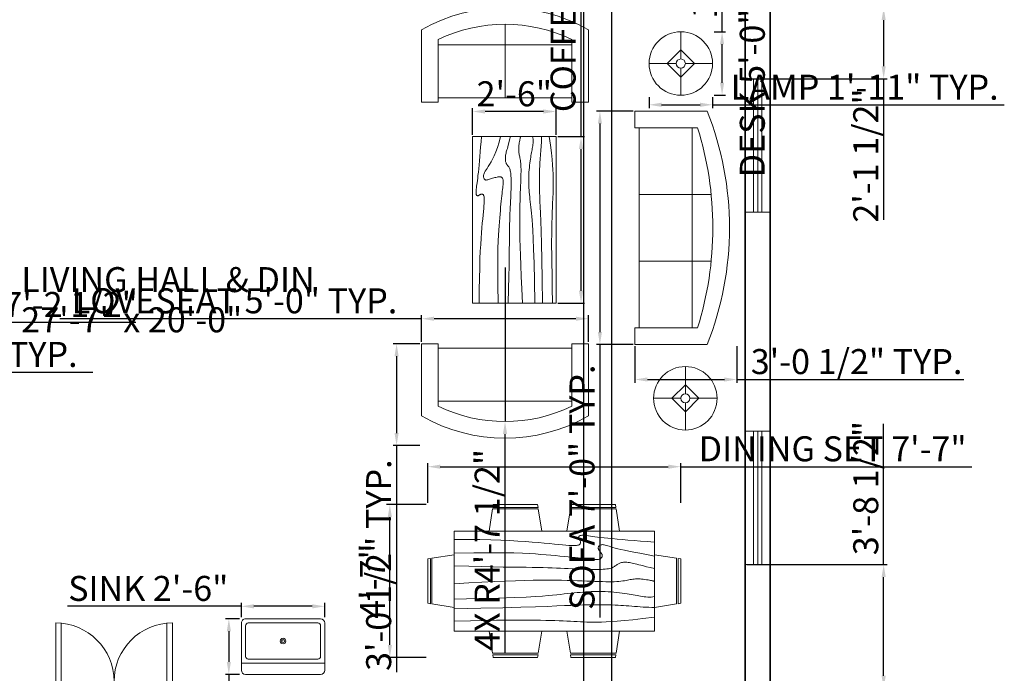
# Model space of a CAD drawing. Units: inches. Extents: x 1885 to 4781, y 1153 to 4395.
# Tile 5 of 7: x 2631 to 2985, y 1789 to 2024. Entities that reach past the tile are written whole.
import ezdxf

# ---------------------------------------------------------------- set-up
doc = ezdxf.new("R2010")
doc.units = ezdxf.units.IN
for name, color, linetype, lineweight in [('A-ANNO-DIMS', 5, 'Continuous', 18), ('A-FURN', 8, 'Continuous', 18), ('A-WALL', 7, 'Continuous', 35)]:
    doc.layers.add(name, color=color, linetype=linetype, lineweight=lineweight)
for name, color, linetype, lineweight, true_color in [('A-AREA-IDEN', 244, 'Continuous', 18, 0x991b1e), ('A-DOOR', 11, 'Continuous', 18, 0xf27172), ('A-FLOR-FIXT', 11, 'Continuous', 18, 0xf27172), ('A-GLAZ', 152, 'Continuous', 18, 0x2776bb)]:
    doc.layers.add(name, color=color, linetype=linetype, lineweight=lineweight, true_color=true_color)
doc.styles.get("Standard").update_dxf_attribs({"font": 'arial.ttf'})
doc.dimstyles.new('ISO-25', dxfattribs={"dimtxt": 9, "dimasz": 4.5, "dimexe": 1.25, "dimexo": 0.625, "dimtad": 1, "dimdec": 0, "dimlunit": 3, "dimtxsty": 'Standard', "dimcen": 2.5, "dimadec": 0, "dimazin": 0, "dimtfac": 1, "dimtdec": 0, "dimtmove": 0, "dimatfit": 3, "dimfxl": 1, "dimarcsym": 0})

# ---------------------------------------------------------------- blocks, each defined once
blk = doc.blocks.new('Table - Rectangular Woodgrain 60 x 30 in.')
for p, q in [((0, 0), (0, -30)), ((60, 0), (0, 0)), ((60, -30), (60, 0)), ((0, -30), (60, -30))]:
    blk.add_line(p, q)
for points in [[(0, -2.4), (4.8155, -2.418), (9.0302, -2.4688), (12.709, -2.5477), (15.9167, -2.65), (18.7181, -2.7711), (21.1781, -2.9063), (23.3616, -3.0508), (25.3333, -3.2), (27.1477, -3.3495), (28.8172, -3.4958), (30.3437, -3.636), (31.7291, -3.7667), (32.9756, -3.8849), (34.0849, -3.9875), (35.059, -4.0714), (35.9, -4.1334), (36.6114, -4.1711), (37.2041, -4.1854), (37.6906, -4.1779), (38.0833, -4.15), (38.3948, -4.1034), (38.6375, -4.0396), (38.8239, -3.9602), (38.9666, -3.8667), (39.0764, -3.7608), (39.1573, -3.6448), (39.2116, -3.521), (39.2416, -3.3917), (39.2498, -3.2593), (39.2385, -3.1261), (39.21, -2.9944), (39.1666, -2.8667), (39.111, -2.7447), (39.0468, -2.6281), (38.978, -2.5163), (38.9083, -2.4083), (38.8418, -2.3035), (38.7823, -2.201), (38.7337, -2.1001), (38.7, -2), (38.6844, -1.9003), (38.6875, -1.8021), (38.7094, -1.707), (38.75, -1.6167), (38.8094, -1.5326), (38.8875, -1.4563), (38.9844, -1.3893), (39.1, -1.3333), (39.2351, -1.2896), (39.3937, -1.2583), (39.5804, -1.2396), (39.8, -1.2333), (40.057, -1.2396), (40.3562, -1.2583), (40.7023, -1.2896), (41.1, -1.3333), (41.5547, -1.3895), (42.0755, -1.4573), (42.6721, -1.5361), (43.3542, -1.625), (44.1316, -1.7233), (45.014, -1.8302), (46.0114, -1.9449), (47.1333, -2.0667), (48.3862, -2.1947), (49.7625, -2.3281), (51.2513, -2.4663), (52.8416, -2.6083), (54.5226, -2.7535), (56.2833, -2.9011), (58.1127, -3.0501), (60, -3.2)], [(0, -9.2), (6.5759, -9.0858), (11.9385, -9.0365), (16.2527, -9.0418), (19.6833, -9.0917), (22.3952, -9.1759), (24.5531, -9.2844), (26.322, -9.4069), (27.8666, -9.5333), (29.3241, -9.6553), (30.7203, -9.7719), (32.0532, -9.8837), (33.3208, -9.9917), (34.5213, -10.0965), (35.6526, -10.199), (36.7128, -10.2999), (37.7, -10.4), (38.6129, -10.4996), (39.4531, -10.5969), (40.223, -10.6895), (40.925, -10.775), (41.5613, -10.8512), (42.1344, -10.9156), (42.6465, -10.966), (43.1, -11), (43.4976, -11.0158), (43.8437, -11.0136), (44.143, -10.9942), (44.4, -10.9583), (44.6195, -10.9069), (44.8062, -10.8406), (44.9648, -10.7603), (45.1, -10.6667), (45.2155, -10.5598), (45.3114, -10.4365), (45.3871, -10.2929), (45.4416, -10.125), (45.4743, -9.929), (45.4844, -9.7011), (45.4709, -9.4371), (45.4333, -9.1333), (45.3716, -8.7883), (45.2896, -8.4104), (45.1919, -8.0107), (45.0833, -7.6), (44.9685, -7.1893), (44.8521, -6.7896), (44.7388, -6.4117), (44.6333, -6.0667), (44.54, -5.7628), (44.4614, -5.4979), (44.4001, -5.2675), (44.3583, -5.0667), (44.3384, -4.8909), (44.3427, -4.7354), (44.3736, -4.5956), (44.4333, -4.4667), (44.5236, -4.3453), (44.6427, -4.2333), (44.7884, -4.1339), (44.9583, -4.05), (45.1501, -3.9849), (45.3614, -3.9417), (45.59, -3.9234), (45.8333, -3.9333), (46.0915, -3.9749), (46.3734, -4.0531), (46.6906, -4.1736), (47.0542, -4.3417), (47.4756, -4.5629), (47.9661, -4.8427), (48.5372, -5.1866), (49.2, -5.6), (49.9676, -6.0844), (50.8594, -6.625), (51.8965, -7.2031), (53.1, -7.8), (54.491, -8.3969), (56.0906, -8.975), (57.9199, -9.5156), (60, -10)], [(0, -12.8), (5.1847, -12.9322), (9.6213, -13.0323), (13.3963, -13.1059), (16.5958, -13.1583), (19.3063, -13.1952), (21.614, -13.2219), (23.6054, -13.2439), (25.3666, -13.2667), (26.9728, -13.2947), (28.4531, -13.3281), (29.8256, -13.3663), (31.1083, -13.4083), (32.3191, -13.4535), (33.476, -13.501), (34.597, -13.5501), (35.7, -13.6), (36.7984, -13.6497), (37.8875, -13.6979), (38.9578, -13.743), (40, -13.7833), (41.0047, -13.8174), (41.9625, -13.8438), (42.864, -13.8607), (43.7, -13.8667), (44.4631, -13.8604), (45.1552, -13.8417), (45.7801, -13.8104), (46.3416, -13.7667), (46.8439, -13.7104), (47.2906, -13.6417), (47.6858, -13.5604), (48.0333, -13.4667), (48.3375, -13.3608), (48.6042, -13.2448), (48.8396, -13.121), (49.05, -12.9917), (49.2417, -12.8593), (49.4208, -12.7261), (49.5937, -12.5944), (49.7667, -12.4667), (49.9452, -12.3451), (50.1323, -12.2313), (50.3303, -12.1268), (50.5416, -12.0333), (50.7686, -11.9524), (51.0135, -11.8854), (51.2788, -11.8341), (51.5666, -11.8), (51.8785, -11.7843), (52.2116, -11.7865), (52.562, -11.8059), (52.926, -11.8417), (53.2998, -11.8931), (53.6795, -11.9594), (54.0614, -12.0397), (54.4416, -12.1333), (54.8223, -12.2401), (55.2293, -12.3625), (55.6942, -12.5037), (56.2489, -12.6667), (56.9251, -12.8547), (57.7545, -13.0708), (58.7689, -13.3182), (60, -13.6)], [(0, -18), (5.124, -17.7273), (9.6609, -17.5057), (13.6705, -17.3303), (17.2125, -17.1958), (20.3467, -17.0973), (23.1328, -17.0297), (25.6307, -16.9878), (27.9, -16.9667), (29.9928, -16.9617), (31.9302, -16.9703), (33.7254, -16.9907), (35.3917, -17.0208), (36.9423, -17.0588), (38.3906, -17.1026), (39.7499, -17.1503), (41.0333, -17.2), (42.2519, -17.2496), (43.4073, -17.2969), (44.4986, -17.3395), (45.525, -17.375), (46.4858, -17.4012), (47.3802, -17.4156), (48.2074, -17.416), (48.9667, -17.4), (49.6583, -17.3662), (50.2872, -17.3167), (50.8595, -17.2547), (51.3812, -17.1833), (51.8584, -17.1057), (52.2971, -17.025), (52.7034, -16.9443), (53.0833, -16.8667), (53.443, -16.7951), (53.789, -16.7313), (54.128, -16.6768), (54.4666, -16.6334), (54.8115, -16.6024), (55.1693, -16.5854), (55.5465, -16.5841), (55.95, -16.6), (56.3828, -16.6337), (56.8346, -16.6823), (57.2915, -16.7418), (57.7396, -16.8084), (58.165, -16.878), (58.5539, -16.9469), (58.8924, -17.0111), (59.1666, -17.0667), (59.3679, -17.1107), (59.5078, -17.1438), (59.6032, -17.1675), (59.6708, -17.1833), (59.7275, -17.193), (59.7901, -17.1979), (59.8753, -17.1998), (60, -17.2)], [(0, -22.4), (8.0098, -22.2501), (14.4094, -22.1011), (19.4168, -21.9535), (23.25, -21.8083), (26.1269, -21.6663), (28.2656, -21.5281), (29.884, -21.3947), (31.2, -21.2667), (32.3967, -21.1448), (33.5172, -21.0292), (34.5697, -20.9198), (35.5625, -20.8167), (36.5037, -20.7198), (37.4015, -20.6292), (38.2642, -20.5448), (39.1, -20.4667), (39.9164, -20.3951), (40.7187, -20.3313), (41.5117, -20.2768), (42.3, -20.2333), (43.0883, -20.2024), (43.8812, -20.1854), (44.6836, -20.1841), (45.5, -20.2), (46.3328, -20.234), (47.1747, -20.2844), (48.0163, -20.3488), (48.8479, -20.425), (49.66, -20.5106), (50.4429, -20.6031), (51.1872, -20.7004), (51.8833, -20.8), (52.5246, -20.8999), (53.1166, -20.9995), (53.6681, -21.0983), (54.1875, -21.1958), (54.6834, -21.2919), (55.1646, -21.3859), (55.6394, -21.4777), (56.1167, -21.5667), (56.6028, -21.6515), (57.0961, -21.7266), (57.5929, -21.7852), (58.0896, -21.8208), (58.5823, -21.8268), (59.0674, -21.7964), (59.5412, -21.723), (60, -21.6)], [(0, -25.2), (8.6355, -25.0504), (15.7026, -24.9031), (21.4049, -24.7606), (25.9458, -24.625), (29.529, -24.4988), (32.3578, -24.3844), (34.6359, -24.284), (36.5667, -24.2), (38.3213, -24.1341), (39.9417, -24.0854), (41.437, -24.0523), (42.8167, -24.0333), (44.0901, -24.0268), (45.2667, -24.0313), (46.3557, -24.0451), (47.3667, -24.0667), (48.309, -24.0947), (49.1928, -24.1287), (50.0284, -24.168), (50.826, -24.2125), (51.5959, -24.2617), (52.3483, -24.3151), (53.0935, -24.3725), (53.8417, -24.4334), (54.6009, -24.497), (55.3699, -24.561), (56.1454, -24.6226), (56.9239, -24.6792), (57.7021, -24.7279), (58.4764, -24.7662), (59.2435, -24.7911), (60, -24.8)], [(0, -28.8), (5.6867, -28.6681), (10.45, -28.5698), (14.407, -28.5012), (17.675, -28.4584), (20.3711, -28.4374), (22.6125, -28.4344), (24.5164, -28.4455), (26.2, -28.4667), (27.762, -28.4947), (29.2276, -28.5281), (30.6033, -28.5663), (31.8958, -28.6084), (33.1118, -28.6535), (34.2578, -28.7011), (35.3405, -28.7501), (36.3666, -28.8), (37.3443, -28.8497), (38.288, -28.8974), (39.2137, -28.9412), (40.1375, -28.9792), (41.0753, -29.0093), (42.0432, -29.0297), (43.0572, -29.0384), (44.1333, -29.0333), (45.2936, -29.0114), (46.5843, -28.9641), (48.0579, -28.8816), (49.7666, -28.7542), (51.7629, -28.5721), (54.0989, -28.3255), (56.8272, -28.0048), (60, -27.6)]]:
    blk.add_lwpolyline(points)
blk = doc.blocks.new('Dining Set - 36 x 72 in.')
for p, q in [((-22.2343, 26.00059), (-23.4847, 17.99762)), ((-22.2304, 26), (-5.7608, 26)), ((-22, 27.5), (-22.1562, 26.50042)), ((-5.8416, 26.5), (-22.1534, 26.5)), ((-22, 27.5), (-6, 27.5)), ((-5.8437, 26.49966), (-6, 27.5)), ((-4.5152, 17.99762), (-5.7655, 25.99926)), ((5.7657, 26.00059), (4.5153, 17.99762)), ((5.7696, 26), (22.2392, 26)), ((6, 27.5), (5.8438, 26.50042)), ((22.1584, 26.5), (5.8466, 26.5)), ((6, 27.5), (22, 27.5)), ((22.1563, 26.49966), (22, 27.5)), ((23.4848, 17.99762), (22.2345, 25.99926)), ((36, 18), (-36, 18)), ((-36, 18), (-36, -18)), ((36, -18), (36, 18)), ((-45.5, 8), (-44.5004, 8.15617)), ((-45.5, 8), (-45.5, -8)), ((-44.5, -8.15843), (-44.5, 8.15338)), ((-44.0006, 8.23428), (-35.9976, 9.48474)), ((-44, 8.23041), (-44, -8.23915)), ((44.0006, 8.23428), (35.9976, 9.48474)), ((44, 8.23041), (44, -8.23915)), ((44.5, -8.15843), (44.5, 8.15338)), ((45.5, 8), (44.5005, 8.15617)), ((45.5, 8), (45.5, -8)), ((-44.4997, -8.15631), (-45.5, -8)), ((-35.9976, -9.48476), (-43.9993, -8.2345)), ((35.9976, -9.48476), (43.9993, -8.2345)), ((44.4997, -8.15631), (45.5, -8)), ((-36, -18), (36, -18)), ((-22.2343, -26.0006), (-23.4847, -17.99762)), ((-4.5152, -17.99762), (-5.7655, -25.99928)), ((5.7657, -26.0006), (4.5153, -17.99762)), ((23.4848, -17.99762), (22.2345, -25.99928)), ((-22.2304, -26), (-5.7608, -26)), ((-22, -27.5), (-22.1562, -26.50044)), ((-5.8416, -26.5), (-22.1534, -26.5)), ((-22, -27.5), (-6, -27.5)), ((-5.8437, -26.49967), (-6, -27.5)), ((5.7696, -26), (22.2392, -26)), ((6, -27.5), (5.8438, -26.50044)), ((22.1584, -26.5), (5.8466, -26.5)), ((6, -27.5), (22, -27.5)), ((22.1563, -26.49967), (22, -27.5))]:
    blk.add_line(p, q)
for points in [[(-36, 15), (-31.1772, 14.97754), (-26.8079, 14.91406), (-22.8538, 14.81543), (-19.276, 14.6875), (-16.0362, 14.53613), (-13.0957, 14.36718), (-10.4159, 14.18652), (-7.9583, 14), (-5.6904, 13.81315), (-3.6035, 13.63021), (-1.6954, 13.45508), (0.0365, 13.29166), (1.5945, 13.14388), (2.9811, 13.01562), (4.1988, 12.9108), (5.25, 12.83333), (6.1393, 12.78613), (6.8802, 12.76823), (7.4883, 12.77767), (7.9792, 12.8125), (8.3685, 12.87077), (8.6719, 12.95052), (8.9049, 13.0498), (9.0833, 13.16666), (9.2205, 13.29899), (9.3216, 13.44401), (9.3895, 13.59879), (9.4271, 13.76041), (9.4373, 13.92594), (9.4232, 14.09245), (9.3875, 14.257), (9.3333, 14.41666), (9.2638, 14.56917), (9.1836, 14.71484), (9.0975, 14.85465), (9.0104, 14.98958), (8.9272, 15.1206), (8.8529, 15.2487), (8.7922, 15.37483), (8.75, 15.5), (8.7305, 15.62467), (8.7344, 15.74739), (8.7617, 15.86621), (8.8125, 15.97916), (8.8867, 16.08431), (8.9844, 16.17968), (9.1055, 16.26334), (9.25, 16.33333), (9.4189, 16.38802), (9.6172, 16.42708), (9.8506, 16.45052), (10.125, 16.45833), (10.4463, 16.45052), (10.8203, 16.42708), (11.2529, 16.38802), (11.75, 16.33333), (12.3184, 16.26318), (12.9694, 16.17838), (13.7151, 16.07991), (14.5677, 15.96875), (15.5395, 15.84586), (16.6426, 15.71224), (17.8893, 15.56884), (19.2917, 15.41666), (20.859, 15.25667), (22.5879, 15.08984), (24.4721, 14.91715), (26.5052, 14.73958), (28.6809, 14.5581), (30.9929, 14.3737), (33.4347, 14.18733), (36, 14)], [(-36, 10), (-28.9766, 10.14274), (-23.1725, 10.20442), (-18.4241, 10.19775), (-14.5677, 10.13541), (-11.4399, 10.03011), (-8.877, 9.89453), (-6.7154, 9.74137), (-4.7917, 9.58333), (-2.9698, 9.43082), (-1.2246, 9.28515), (0.4415, 9.14534), (2.026, 9.01041), (3.5266, 8.87939), (4.9408, 8.7513), (6.266, 8.62516), (7.5, 8.5), (8.6411, 8.37549), (9.6914, 8.2539), (10.6538, 8.13818), (11.5312, 8.03125), (12.3267, 7.93603), (13.043, 7.85547), (13.6831, 7.79248), (14.25, 7.75), (14.7471, 7.7303), (15.1797, 7.73307), (15.5537, 7.75732), (15.875, 7.80208), (16.1494, 7.86637), (16.3828, 7.94922), (16.5811, 8.04964), (16.75, 8.16666), (16.8944, 8.29915), (17.0143, 8.44531), (17.1089, 8.60319), (17.1771, 8.77083), (17.218, 8.94629), (17.2305, 9.1276), (17.2137, 9.31282), (17.1667, 9.5), (17.0895, 9.6875), (16.987, 9.875), (16.8649, 10.0625), (16.7292, 10.25), (16.5856, 10.4375), (16.4401, 10.625), (16.2985, 10.8125), (16.1667, 11), (16.05, 11.18733), (15.9518, 11.3737), (15.8752, 11.5581), (15.8229, 11.73958), (15.798, 11.91715), (15.8034, 12.08984), (15.842, 12.25667), (15.9167, 12.41666), (16.0295, 12.56836), (16.1784, 12.70833), (16.3605, 12.83268), (16.5729, 12.9375), (16.8127, 13.01888), (17.0768, 13.07291), (17.3625, 13.0957), (17.6667, 13.08333), (17.9894, 13.03312), (18.3418, 12.94726), (18.7382, 12.82918), (19.1927, 12.68229), (19.7195, 12.51001), (20.3327, 12.31575), (21.0465, 12.10294), (21.875, 11.875), (22.8357, 11.63354), (23.959, 11.37304), (25.2786, 11.08618), (26.8282, 10.76562), (28.6414, 10.40405), (30.752, 9.99414), (33.1936, 9.52856), (36, 9)], [(-36, 5.5), (-30.7157, 5.3348), (-26.069, 5.20963), (-21.9946, 5.11767), (-18.4271, 5.05208), (-15.3009, 5.00602), (-12.5508, 4.97265), (-10.1112, 4.94515), (-7.9167, 4.91666), (-5.909, 4.88167), (-4.0586, 4.83984), (-2.3429, 4.79215), (-0.7396, 4.73958), (0.7739, 4.6831), (2.22, 4.6237), (3.6213, 4.56233), (5, 4.5), (6.373, 4.43782), (7.7344, 4.3776), (9.0723, 4.32129), (10.375, 4.27083), (11.6309, 4.22819), (12.8281, 4.19531), (13.9551, 4.17415), (15, 4.16666), (15.954, 4.17448), (16.819, 4.19791), (17.6001, 4.23698), (18.3021, 4.29166), (18.9299, 4.36198), (19.4883, 4.44791), (19.9823, 4.54948), (20.4167, 4.66666), (20.7969, 4.79899), (21.1302, 4.94401), (21.4245, 5.09879), (21.6875, 5.26041), (21.9271, 5.42594), (22.1511, 5.59245), (22.3672, 5.757), (22.5834, 5.91666), (22.8065, 6.06868), (23.0404, 6.21093), (23.2879, 6.34147), (23.5521, 6.45833), (23.8358, 6.55957), (24.142, 6.64323), (24.4735, 6.70735), (24.8334, 6.75), (25.2235, 6.76969), (25.642, 6.76692), (26.0858, 6.74267), (26.5521, 6.69791), (27.0379, 6.63362), (27.5404, 6.55078), (28.0565, 6.45036), (28.5834, 6.33333), (29.1242, 6.19987), (29.7071, 6.04687), (30.3661, 5.87044), (31.1354, 5.66666), (32.0493, 5.43164), (33.142, 5.16146), (34.4475, 4.85221), (36, 4.5)], [(-36, -1), (-30.7915, -0.6591), (-26.0195, -0.38216), (-21.6519, -0.16284), (-17.6563, 0.00521), (-14.0005, 0.12833), (-10.6523, 0.21289), (-7.5796, 0.26522), (-4.75, 0.29166), (-2.134, 0.29793), (0.2878, 0.28711), (2.5317, 0.26163), (4.6146, 0.22396), (6.5529, 0.17651), (8.3633, 0.12174), (10.0623, 0.06209), (11.6667, 0), (13.1899, -0.06201), (14.6341, -0.1211), (15.9982, -0.17432), (17.2813, -0.21875), (18.4823, -0.25147), (19.6003, -0.26953), (20.6343, -0.27002), (21.5834, -0.25), (22.4481, -0.20768), (23.2357, -0.14584), (23.9549, -0.06836), (24.6146, 0.02083), (25.2235, 0.11784), (25.7904, 0.21875), (26.3241, 0.31966), (26.8334, 0.41666), (27.3265, 0.50618), (27.8099, 0.58593), (28.2894, 0.65397), (28.7709, 0.70833), (29.2601, 0.74707), (29.763, 0.76823), (30.2855, 0.76985), (30.8334, 0.75), (31.4088, 0.70784), (31.9994, 0.64713), (32.589, 0.57275), (33.1615, 0.48958), (33.7008, 0.4025), (34.1908, 0.3164), (34.6153, 0.23616), (34.9584, 0.16666), (35.2099, 0.11165), (35.3848, 0.07031), (35.504, 0.04069), (35.5886, 0.02083), (35.6594, 0.00879), (35.7377, 0.0026), (35.8442, 0.00032), (36, 0)], [(-36, -6.5), (-27.1843, -6.31267), (-20.084, -6.1263), (-14.469, -5.9419), (-10.1094, -5.76042), (-6.7752, -5.58285), (-4.2363, -5.41016), (-2.2629, -5.24333), (-0.625, -5.08334), (0.8708, -4.93099), (2.2715, -4.78646), (3.5872, -4.64974), (4.8281, -4.52084), (6.0046, -4.39974), (7.127, -4.28646), (8.2053, -4.18099), (9.25, -4.08334), (10.2705, -3.99382), (11.2734, -3.91407), (12.2647, -3.84603), (13.25, -3.79167), (14.2354, -3.75293), (15.2266, -3.73177), (16.2295, -3.73015), (17.25, -3.75), (18.2912, -3.79248), (19.3451, -3.85547), (20.4009, -3.93604), (21.4479, -4.03125), (22.4754, -4.13819), (23.4727, -4.25391), (24.4289, -4.37549), (25.3334, -4.5), (26.1785, -4.62492), (26.9694, -4.74935), (27.7145, -4.87281), (28.4219, -4.99479), (29.1, -5.11483), (29.7572, -5.23242), (30.4016, -5.34709), (31.0417, -5.45834), (31.6837, -5.56437), (32.3262, -5.65821), (32.9658, -5.73153), (33.599, -5.77604), (34.2224, -5.78345), (34.8327, -5.74545), (35.4264, -5.65373), (36, -5.5)], [(-36, -10), (-26.4022, -9.81299), (-18.4675, -9.62891), (-11.9839, -9.45069), (-6.7396, -9.28125), (-2.5226, -9.12354), (0.8789, -8.98047), (3.6769, -8.85498), (6.0833, -8.75), (8.2767, -8.66765), (10.3021, -8.60677), (12.1712, -8.56543), (13.8958, -8.54167), (15.4876, -8.53353), (16.9583, -8.53907), (18.3197, -8.55632), (19.5834, -8.58334), (20.7616, -8.61841), (21.8685, -8.66081), (22.9188, -8.71004), (23.9271, -8.76563), (24.9081, -8.82707), (25.8763, -8.89388), (26.8465, -8.96558), (27.8334, -9.04167), (28.8474, -9.12118), (29.8828, -9.20117), (30.93, -9.27824), (31.9792, -9.34896), (33.0205, -9.40991), (34.0443, -9.45768), (35.0407, -9.48885), (36, -9.5)], [(-36, -14.5), (-30.0881, -14.33513), (-25.0332, -14.21224), (-20.7312, -14.12647), (-17.0781, -14.07292), (-13.97, -14.04671), (-11.3027, -14.04297), (-8.9724, -14.05681), (-6.875, -14.08334), (-4.9224, -14.11833), (-3.0905, -14.16016), (-1.3709, -14.20785), (0.2448, -14.26042), (1.7647, -14.3169), (3.1973, -14.3763), (4.5507, -14.43767), (5.8333, -14.5), (7.0554, -14.5621), (8.235, -14.62175), (9.3922, -14.67652), (10.5469, -14.72396), (11.7192, -14.76164), (12.929, -14.78711), (14.1965, -14.79794), (15.5417, -14.79167), (16.9933, -14.76424), (18.6152, -14.70508), (20.4804, -14.60197), (22.6615, -14.44271), (25.2312, -14.21509), (28.2624, -13.9069), (31.8277, -13.50594), (36, -13)]]:
    blk.add_lwpolyline(points)
blk = doc.blocks.new('Lamp - Table')
for p, q in [((0, 7), (0, 1)), ((0, 3), (-3, 0)), ((3, 0), (0, 3)), ((-1, 0), (-7, 0)), ((-3, 0), (0, -3)), ((0, -3), (3, 0)), ((1, 0), (7, 0)), ((0, -1), (0, -7))]:
    blk.add_line(p, q)
for radius in [7, 1]:
    blk.add_circle((0, 0), radius)
blk = doc.blocks.new('Sofa - Roundback Loveseat 5 ft.')
for p, q in [((0, -32.44198), (0, -5.99998)), ((-24, -33.99998), (-24, -11.46958)), ((-23.9998, -13.38178), (23.99986, -13.38178)), ((24.00004, -33.99998), (24.00004, -11.46958)), ((-24, -32.44198), (24.00004, -32.44198))]:
    blk.add_line(p, q)
for points in [[(-24, -33.99998), (-30, -33.99998), (-30, -7.99998)], [(30.00004, -7.99998), (30.00004, -33.99998), (24.00004, -33.99998)]]:
    blk.add_lwpolyline(points)
for centre, radius, start, end in [((0, -60.24998), 60.24998, 60.13715, 119.8628), ((0, -61.38438), 55.38444, 64.32083, 115.6792)]:
    blk.add_arc(centre, radius, start, end)
blk = doc.blocks.new('Sofa - Roundback 7 ft.')
for p, q in [((-12.00002, -32.4421), (-12.00003, -6.5971)), ((11.99997, -32.4421), (11.99998, -6.5971)), ((-36.000027, -34), (-36.000027, -11.4696)), ((-35.999844, -13.3819), (35.9998, -13.3819)), ((35.99998, -34), (35.99998, -11.4696)), ((-36.000027, -32.4421), (35.99998, -32.4421))]:
    blk.add_line(p, q)
for points in [[(-36.000027, -34), (-42.000027, -34), (-42.000027, -8)], [(41.99998, -8), (41.99998, -34), (35.99998, -34)]]:
    blk.add_lwpolyline(points)
for centre, radius, start, end in [((0, -114.25), 114.25, 68.43141, 111.5686), ((-0.00001, -127.1968), 121.1968, 72.72033, 107.2797)]:
    blk.add_arc(centre, radius, start, end)
blk = doc.blocks.new('Sink-single - 30 in top')
blk.add_line((-15, -3.999996), (15, -3.999996))
for points in [[(-13.5, 0), (13.5, 0)], [(-15, -18.499996), (-15, -1.5)], [(15, -1.5), (15, -18.499996)], [(-13.5, -17.499996), (-13.5, -6.499996)], [(-12.5, -5.499996), (12.5, -5.499996)], [(13.5, -6.499996), (13.5, -17.499996)], [(13.5, -19.999996), (-13.5, -19.999996)], [(12.5, -18.499996), (-12.5, -18.499996)]]:
    blk.add_lwpolyline(points)
for radius in [1, 0.5]:
    blk.add_circle((0, -11.999996), radius)
for centre, radius, start, end in [((-13.5, -1.5), 1.5, 90, 180), ((13.5, -1.5), 1.5, 0, 90), ((-12.5, -6.499996), 1, 90, 180), ((12.5, -6.499996), 1, 0, 90), ((-12.5, -17.499996), 1, 180, 270), ((12.5, -17.499996), 1, 270, 0), ((-13.5, -18.499996), 1.5, 180, 270), ((13.5, -18.499996), 1.5, 270, 0)]:
    blk.add_arc(centre, radius, start, end)
blk = doc.blocks.new('WIN-48IN')
for p, q in [((0, 9), (48, 9)), ((0, 0), (0, 9)), ((48, 9), (48, 0)), ((0, 6), (48, 6)), ((0, 4.5), (48, 4.5)), ((0, 3), (48, 3)), ((48, 0), (0, 0))]:
    blk.add_line(p, q)
blk = doc.blocks.new('DOOR-PAIR-42IN')
for p, q in [((0, 21), (0, 0)), ((2, 21), (2, 0)), ((40, 21), (40, 0)), ((42, 21), (42, 0)), ((0, 0), (2, 0)), ((42, 0), (40, 0))]:
    blk.add_line(p, q)
for centre, start, end in [((0, 0), 0, 90), ((42, 0), 90, 180)]:
    blk.add_arc(centre, 21, start, end)
blk = doc.blocks.new('*D35')
at = {"layer": 'A-ANNO-DIMS', "color": 0, "lineweight": -2, "transparency": 16777216}
for p, q in [((2857.33, 1996.23), (2857.33, 1992.18)), ((2880.17, 1996.23), (2880.17, 1992.18)), ((2861.83, 1993.43), (2875.67, 1993.43)), ((2880.17, 1993.43), (2985.1, 1993.43))]:
    blk.add_line(p, q, dxfattribs=at)
at = {"layer": 'A-ANNO-DIMS', "color": 0, "transparency": 16777216}
for points in [[(2861.83, 1994.18), (2861.83, 1992.68), (2857.33, 1993.43)], [(2875.67, 1994.18), (2875.67, 1992.68), (2880.17, 1993.43)]]:
    blk.add_solid(points, dxfattribs=at)
at = {"layer": 'Defpoints', "color": 0, "transparency": 16777216}
for p in [(2857.33, 1996.86), (2880.17, 1996.86), (2880.17, 1993.43)]:
    blk.add_point(p, dxfattribs=at)
at = {"layer": 'A-ANNO-DIMS', "color": 0, "transparency": 16777216, "insert": (2934.88, 1998.58), "char_height": 9, "attachment_point": 5}
blk.add_mtext('LAMP 1\'-11" TYP.', dxfattribs=at)
blk = doc.blocks.new('*D36')
at = {"layer": 'A-ANNO-DIMS', "color": 0, "lineweight": -2, "transparency": 16777216}
for p, q in [((2883.59, 2019.7), (2883.59, 2086.45)), ((2880.79, 2019.7), (2884.84, 2019.7)), ((2883.59, 2001.36), (2883.59, 2015.2)), ((2880.79, 1996.86), (2884.84, 1996.86))]:
    blk.add_line(p, q, dxfattribs=at)
at = {"layer": 'A-ANNO-DIMS', "color": 0, "transparency": 16777216}
for points in [[(2882.84, 2015.2), (2884.34, 2015.2), (2883.59, 2019.7)], [(2882.84, 2001.36), (2884.34, 2001.36), (2883.59, 1996.86)]]:
    blk.add_solid(points, dxfattribs=at)
at = {"layer": 'Defpoints', "color": 0, "transparency": 16777216}
for p in [(2880.17, 2019.7), (2883.59, 2019.7), (2880.17, 1996.86)]:
    blk.add_point(p, dxfattribs=at)
at = {"layer": 'A-ANNO-DIMS', "color": 0, "transparency": 16777216, "insert": (2878.45, 2055.33), "char_height": 9, "attachment_point": 5, "rotation": 90}
blk.add_mtext('1\'-11" TYP.', dxfattribs=at)
blk = doc.blocks.new('*D39')
at = {"layer": 'A-ANNO-DIMS', "color": 0, "lineweight": -2, "transparency": 16777216}
for p, q in [((2851.64, 1991.15), (2838.41, 1991.15)), ((2839.66, 1986.65), (2839.66, 1911.65)), ((2851.64, 1907.15), (2838.41, 1907.15)), ((2839.66, 1907.15), (2839.66, 1808.86))]:
    blk.add_line(p, q, dxfattribs=at)
at = {"layer": 'A-ANNO-DIMS', "color": 0, "transparency": 16777216}
for points in [[(2838.91, 1986.65), (2840.41, 1986.65), (2839.66, 1991.15)], [(2838.91, 1911.65), (2840.41, 1911.65), (2839.66, 1907.15)]]:
    blk.add_solid(points, dxfattribs=at)
at = {"layer": 'Defpoints', "color": 0, "transparency": 16777216}
for p in [(2852.26, 1991.15), (2839.66, 1907.15), (2852.26, 1907.15)]:
    blk.add_point(p, dxfattribs=at)
at = {"layer": 'A-ANNO-DIMS', "color": 0, "transparency": 16777216, "insert": (2834.38, 1855.76), "char_height": 9, "attachment_point": 5, "rotation": 90}
blk.add_mtext('SOFA 7\'-0" TYP.', dxfattribs=at)
blk = doc.blocks.new('*D40')
at = {"layer": 'A-ANNO-DIMS', "color": 0, "lineweight": -2, "transparency": 16777216}
for p, q in [((2852.26, 1906.53), (2852.26, 1893.3)), ((2888.93, 1906.53), (2888.93, 1893.3)), ((2856.76, 1894.55), (2884.43, 1894.55)), ((2888.93, 1894.55), (2970.5, 1894.55))]:
    blk.add_line(p, q, dxfattribs=at)
at = {"layer": 'A-ANNO-DIMS', "color": 0, "transparency": 16777216}
for points in [[(2856.76, 1895.3), (2856.76, 1893.8), (2852.26, 1894.55)], [(2884.43, 1895.3), (2884.43, 1893.8), (2888.93, 1894.55)]]:
    blk.add_solid(points, dxfattribs=at)
at = {"layer": 'Defpoints', "color": 0, "transparency": 16777216}
for p in [(2852.26, 1907.15), (2888.93, 1907.15), (2888.93, 1894.55)]:
    blk.add_point(p, dxfattribs=at)
at = {"layer": 'A-ANNO-DIMS', "color": 0, "transparency": 16777216, "insert": (2931.97, 1899.84), "char_height": 9, "attachment_point": 5}
blk.add_mtext('3\'-0 1/2" TYP.', dxfattribs=at)
blk = doc.blocks.new('*D43')
at = {"layer": 'A-ANNO-DIMS', "color": 0, "lineweight": -2, "transparency": 16777216}
for p, q in [((2775.52, 1916.43), (2645.44, 1916.43)), ((2775.52, 1908.06), (2775.52, 1917.68)), ((2831.02, 1916.43), (2780.02, 1916.43)), ((2835.52, 1908.06), (2835.52, 1917.68))]:
    blk.add_line(p, q, dxfattribs=at)
at = {"layer": 'A-ANNO-DIMS', "color": 0, "transparency": 16777216}
for points in [[(2780.02, 1917.18), (2780.02, 1915.68), (2775.52, 1916.43)], [(2831.02, 1917.18), (2831.02, 1915.68), (2835.52, 1916.43)]]:
    blk.add_solid(points, dxfattribs=at)
at = {"layer": 'Defpoints', "color": 0, "transparency": 16777216}
for p in [(2775.52, 1916.43), (2775.52, 1907.43), (2835.52, 1907.43)]:
    blk.add_point(p, dxfattribs=at)
at = {"layer": 'A-ANNO-DIMS', "color": 0, "transparency": 16777216, "insert": (2708.23, 1921.72), "char_height": 9, "attachment_point": 5}
blk.add_mtext('LOVESEAT 5\'-0" TYP.', dxfattribs=at)
blk = doc.blocks.new('*D44')
at = {"layer": 'A-ANNO-DIMS', "color": 0, "lineweight": -2, "transparency": 16777216}
for p, q in [((2774.9, 1907.43), (2765.27, 1907.43)), ((2766.52, 1902.93), (2766.52, 1875.27)), ((2774.9, 1870.77), (2765.27, 1870.77)), ((2766.52, 1870.77), (2766.52, 1789.19))]:
    blk.add_line(p, q, dxfattribs=at)
at = {"layer": 'A-ANNO-DIMS', "color": 0, "transparency": 16777216}
for points in [[(2765.77, 1902.93), (2767.27, 1902.93), (2766.52, 1907.43)], [(2765.77, 1875.27), (2767.27, 1875.27), (2766.52, 1870.77)]]:
    blk.add_solid(points, dxfattribs=at)
at = {"layer": 'Defpoints', "color": 0, "transparency": 16777216}
for p in [(2775.52, 1907.43), (2766.52, 1870.77), (2775.52, 1870.77)]:
    blk.add_point(p, dxfattribs=at)
at = {"layer": 'A-ANNO-DIMS', "color": 0, "transparency": 16777216, "insert": (2761.24, 1827.73), "char_height": 9, "attachment_point": 5, "rotation": 90}
blk.add_mtext('3\'-0 1/2" TYP.', dxfattribs=at)
blk = doc.blocks.new('*D57')
at = {"layer": 'A-ANNO-DIMS', "color": 0, "lineweight": -2, "transparency": 16777216}
for p, q in [((2465.66, 1891.47), (2465.66, 1898.39)), ((2507.66, 1891.47), (2507.66, 1898.39)), ((2470.16, 1897.14), (2503.16, 1897.14)), ((2507.66, 1897.14), (2657.22, 1897.14))]:
    blk.add_line(p, q, dxfattribs=at)
at = {"layer": 'A-ANNO-DIMS', "color": 0, "transparency": 16777216}
for points in [[(2470.16, 1897.89), (2470.16, 1896.39), (2465.66, 1897.14)], [(2503.16, 1897.89), (2503.16, 1896.39), (2507.66, 1897.14)]]:
    blk.add_solid(points, dxfattribs=at)
at = {"layer": 'Defpoints', "color": 0, "transparency": 16777216}
for p in [(2507.66, 1897.14), (2465.66, 1890.84), (2507.66, 1890.84)]:
    blk.add_point(p, dxfattribs=at)
at = {"layer": 'A-ANNO-DIMS', "color": 0, "transparency": 16777216, "insert": (2584.69, 1902.43), "char_height": 9, "attachment_point": 5}
blk.add_mtext('RUG CORNER 3\'-6" TYP.', dxfattribs=at)
blk = doc.blocks.new('*D59')
at = {"layer": 'A-ANNO-DIMS', "color": 0, "lineweight": -2, "transparency": 16777216}
for p, q in [((2832.86, 1982.01), (2832.86, 2109.39)), ((2824.49, 1982.01), (2834.11, 1982.01)), ((2832.86, 1926.51), (2832.86, 1977.51)), ((2824.49, 1922.01), (2834.11, 1922.01))]:
    blk.add_line(p, q, dxfattribs=at)
at = {"layer": 'A-ANNO-DIMS', "color": 0, "transparency": 16777216}
for points in [[(2832.11, 1977.51), (2833.61, 1977.51), (2832.86, 1982.01)], [(2832.11, 1926.51), (2833.61, 1926.51), (2832.86, 1922.01)]]:
    blk.add_solid(points, dxfattribs=at)
at = {"layer": 'Defpoints', "color": 0, "transparency": 16777216}
for p in [(2823.86, 1982.01), (2832.86, 1982.01), (2823.86, 1922.01)]:
    blk.add_point(p, dxfattribs=at)
at = {"layer": 'A-ANNO-DIMS', "color": 0, "transparency": 16777216, "insert": (2827.58, 2047.95), "char_height": 9, "attachment_point": 5, "rotation": 90}
blk.add_mtext('COFFEE TABLE 5\'-0"', dxfattribs=at)
blk = doc.blocks.new('*D60')
at = {"layer": 'A-ANNO-DIMS', "color": 0, "lineweight": -2, "transparency": 16777216}
for p, q in [((2793.86, 1982.64), (2793.86, 1992.26)), ((2819.36, 1991.01), (2798.36, 1991.01)), ((2823.86, 1982.64), (2823.86, 1992.26))]:
    blk.add_line(p, q, dxfattribs=at)
at = {"layer": 'A-ANNO-DIMS', "color": 0, "transparency": 16777216}
for points in [[(2798.36, 1991.76), (2798.36, 1990.26), (2793.86, 1991.01)], [(2819.36, 1991.76), (2819.36, 1990.26), (2823.86, 1991.01)]]:
    blk.add_solid(points, dxfattribs=at)
at = {"layer": 'Defpoints', "color": 0, "transparency": 16777216}
for p in [(2793.86, 1991.01), (2793.86, 1982.01), (2823.86, 1982.01)]:
    blk.add_point(p, dxfattribs=at)
at = {"layer": 'A-ANNO-DIMS', "color": 0, "transparency": 16777216, "insert": (2808.86, 1996.23), "char_height": 9, "attachment_point": 5}
blk.add_mtext('2\'-6"', dxfattribs=at)
blk = doc.blocks.new('*D63')
at = {"layer": 'A-ANNO-DIMS', "color": 0, "lineweight": -2, "transparency": 16777216}
for p, q in [((2777.75, 1850.14), (2777.75, 1864.42)), ((2782.25, 1863.17), (2864.25, 1863.17)), ((2868.75, 1850.14), (2868.75, 1864.42)), ((2868.75, 1863.17), (2973.42, 1863.17))]:
    blk.add_line(p, q, dxfattribs=at)
at = {"layer": 'A-ANNO-DIMS', "color": 0, "transparency": 16777216}
for points in [[(2782.25, 1863.92), (2782.25, 1862.42), (2777.75, 1863.17)], [(2864.25, 1863.92), (2864.25, 1862.42), (2868.75, 1863.17)]]:
    blk.add_solid(points, dxfattribs=at)
at = {"layer": 'Defpoints', "color": 0, "transparency": 16777216}
for p in [(2868.75, 1863.17), (2777.75, 1849.52), (2868.75, 1849.52)]:
    blk.add_point(p, dxfattribs=at)
at = {"layer": 'A-ANNO-DIMS', "color": 0, "transparency": 16777216, "insert": (2923.34, 1868.45), "char_height": 9, "attachment_point": 5}
blk.add_mtext('DINING SET 7\'-7"', dxfattribs=at)
blk = doc.blocks.new('*D64')
at = {"layer": 'A-ANNO-DIMS', "color": 0, "lineweight": -2, "transparency": 16777216}
for p, q in [((2777.13, 1849.52), (2762.85, 1849.52)), ((2764.1, 1799.02), (2764.1, 1845.02)), ((2777.13, 1794.52), (2762.85, 1794.52))]:
    blk.add_line(p, q, dxfattribs=at)
at = {"layer": 'A-ANNO-DIMS', "color": 0, "transparency": 16777216}
for points in [[(2763.35, 1845.02), (2764.85, 1845.02), (2764.1, 1849.52)], [(2763.35, 1799.02), (2764.85, 1799.02), (2764.1, 1794.52)]]:
    blk.add_solid(points, dxfattribs=at)
at = {"layer": 'Defpoints', "color": 0, "transparency": 16777216}
for p in [(2764.1, 1849.52), (2777.75, 1849.52), (2777.75, 1794.52)]:
    blk.add_point(p, dxfattribs=at)
at = {"layer": 'A-ANNO-DIMS', "color": 0, "transparency": 16777216, "insert": (2758.98, 1822.02), "char_height": 9, "attachment_point": 5, "rotation": 90}
blk.add_mtext('4\'-7"', dxfattribs=at)
blk = doc.blocks.new('*D71')
at = {"layer": 'A-ANNO-DIMS', "color": 0, "lineweight": -2, "transparency": 16777216}
for p, q in [((2710.69, 1809.05), (2710.69, 1814.17)), ((2740.69, 1809.05), (2740.69, 1814.17)), ((2710.69, 1812.92), (2648.22, 1812.92)), ((2736.19, 1812.92), (2715.19, 1812.92))]:
    blk.add_line(p, q, dxfattribs=at)
at = {"layer": 'A-ANNO-DIMS', "color": 0, "transparency": 16777216}
for points in [[(2715.19, 1813.67), (2715.19, 1812.17), (2710.69, 1812.92)], [(2736.19, 1813.67), (2736.19, 1812.17), (2740.69, 1812.92)]]:
    blk.add_solid(points, dxfattribs=at)
at = {"layer": 'Defpoints', "color": 0, "transparency": 16777216}
for p in [(2710.69, 1812.92), (2710.69, 1808.42), (2740.69, 1808.42)]:
    blk.add_point(p, dxfattribs=at)
at = {"layer": 'A-ANNO-DIMS', "color": 0, "transparency": 16777216, "insert": (2677.21, 1818.2), "char_height": 9, "attachment_point": 5}
blk.add_mtext('SINK 2\'-6"', dxfattribs=at)
blk = doc.blocks.new('*D72')
at = {"layer": 'A-ANNO-DIMS', "color": 0, "lineweight": -2, "transparency": 16777216}
for p, q in [((2710.07, 1808.42), (2704.94, 1808.42)), ((2706.19, 1803.92), (2706.19, 1792.92)), ((2710.07, 1788.42), (2704.94, 1788.42)), ((2706.19, 1788.42), (2706.19, 1759.59))]:
    blk.add_line(p, q, dxfattribs=at)
at = {"layer": 'A-ANNO-DIMS', "color": 0, "transparency": 16777216}
for points in [[(2705.44, 1803.92), (2706.94, 1803.92), (2706.19, 1808.42)], [(2705.44, 1792.92), (2706.94, 1792.92), (2706.19, 1788.42)]]:
    blk.add_solid(points, dxfattribs=at)
at = {"layer": 'Defpoints', "color": 0, "transparency": 16777216}
for p in [(2710.69, 1808.42), (2706.19, 1788.42), (2710.69, 1788.42)]:
    blk.add_point(p, dxfattribs=at)
at = {"layer": 'A-ANNO-DIMS', "color": 0, "transparency": 16777216, "insert": (2700.97, 1771.76), "char_height": 9, "attachment_point": 5, "rotation": 90}
blk.add_mtext('1\'-8"', dxfattribs=at)
blk = doc.blocks.new('*D73')
at = {"layer": 'A-ANNO-DIMS', "color": 0, "lineweight": -2, "transparency": 16777216}
for p, q in [((2892.53, 2093.42), (2902.16, 2093.42)), ((2900.91, 2088.92), (2900.91, 2037.92)), ((2892.53, 2033.42), (2902.16, 2033.42)), ((2900.91, 2033.42), (2900.91, 1966.46))]:
    blk.add_line(p, q, dxfattribs=at)
at = {"layer": 'A-ANNO-DIMS', "color": 0, "transparency": 16777216}
for points in [[(2900.16, 2088.92), (2901.66, 2088.92), (2900.91, 2093.42)], [(2900.16, 2037.92), (2901.66, 2037.92), (2900.91, 2033.42)]]:
    blk.add_solid(points, dxfattribs=at)
at = {"layer": 'Defpoints', "color": 0, "transparency": 16777216}
for p in [(2891.91, 2093.42), (2891.91, 2033.42), (2900.91, 2033.42)]:
    blk.add_point(p, dxfattribs=at)
at = {"layer": 'A-ANNO-DIMS', "color": 0, "transparency": 16777216, "insert": (2895.63, 1997.69), "char_height": 9, "attachment_point": 5, "rotation": 90}
blk.add_mtext('DESK 5\'-0"', dxfattribs=at)
blk = doc.blocks.new('*D88')
at = {"layer": 'A-ANNO-DIMS', "color": 0, "lineweight": -2, "transparency": 16777216}
for p, q in [((2892.53, 2028.42), (2942.96, 2028.42)), ((2941.71, 2023.92), (2941.71, 2007.32)), ((2892.53, 2002.82), (2942.96, 2002.82)), ((2941.71, 2002.82), (2941.71, 1952.02))]:
    blk.add_line(p, q, dxfattribs=at)
at = {"layer": 'A-ANNO-DIMS', "color": 0, "transparency": 16777216}
for points in [[(2940.96, 2023.92), (2942.46, 2023.92), (2941.71, 2028.42)], [(2940.96, 2007.32), (2942.46, 2007.32), (2941.71, 2002.82)]]:
    blk.add_solid(points, dxfattribs=at)
at = {"layer": 'Defpoints', "color": 0, "transparency": 16777216}
for p in [(2891.91, 2028.42), (2891.91, 2002.82), (2941.71, 2002.82)]:
    blk.add_point(p, dxfattribs=at)
at = {"layer": 'A-ANNO-DIMS', "color": 0, "transparency": 16777216, "insert": (2936.43, 1975.17), "char_height": 9, "attachment_point": 5, "rotation": 90}
blk.add_mtext('2\'-1 1/2"', dxfattribs=at)
blk = doc.blocks.new('*D89')
at = {"layer": 'A-ANNO-DIMS', "color": 0, "lineweight": -2, "transparency": 16777216}
for p, q in [((2941.71, 1827.92), (2941.71, 1878.56)), ((2892.53, 1827.92), (2942.96, 1827.92)), ((2941.71, 1787.92), (2941.71, 1823.42)), ((2892.53, 1783.42), (2942.96, 1783.42))]:
    blk.add_line(p, q, dxfattribs=at)
at = {"layer": 'A-ANNO-DIMS', "color": 0, "transparency": 16777216}
for points in [[(2940.96, 1823.42), (2942.46, 1823.42), (2941.71, 1827.92)], [(2940.96, 1787.92), (2942.46, 1787.92), (2941.71, 1783.42)]]:
    blk.add_solid(points, dxfattribs=at)
at = {"layer": 'Defpoints', "color": 0, "transparency": 16777216}
for p in [(2891.91, 1827.92), (2941.71, 1827.92), (2891.91, 1783.42)]:
    blk.add_point(p, dxfattribs=at)
at = {"layer": 'A-ANNO-DIMS', "color": 0, "transparency": 16777216, "insert": (2936.43, 1855.49), "char_height": 9, "attachment_point": 5, "rotation": 90}
blk.add_mtext('3\'-8 1/2"', dxfattribs=at)
blk = doc.blocks.new('*D92')
at = {"layer": 'A-ANNO-DIMS', "color": 0, "lineweight": -2, "transparency": 16777216}
for p, q in [((2829.41, 2263.22), (2824.91, 2263.22)), ((2833.91, 1724.05), (2833.91, 2264.47)), ((2833.91, 2263.22), (2843.91, 2263.22)), ((2843.91, 1724.05), (2843.91, 2264.47)), ((2848.41, 2263.22), (2885.07, 2263.22))]:
    blk.add_line(p, q, dxfattribs=at)
at = {"layer": 'A-ANNO-DIMS', "color": 0, "transparency": 16777216}
for points in [[(2829.41, 2263.97), (2829.41, 2262.47), (2833.91, 2263.22)], [(2848.41, 2263.97), (2848.41, 2262.47), (2843.91, 2263.22)]]:
    blk.add_solid(points, dxfattribs=at)
at = {"layer": 'Defpoints', "color": 0, "transparency": 16777216}
for p in [(2843.91, 2263.22), (2833.91, 1723.42), (2843.91, 1723.42)]:
    blk.add_point(p, dxfattribs=at)
at = {"layer": 'A-ANNO-DIMS', "color": 0, "transparency": 16777216, "insert": (2868.99, 2268.44), "char_height": 9, "attachment_point": 5}
blk.add_mtext('0\'-10"', dxfattribs=at)
blk = doc.blocks.new('*D96')
at = {"layer": 'A-ANNO-DIMS', "color": 0, "lineweight": -2, "transparency": 16777216}
for p, q in [((2805.52, 1934.82), (2805.52, 1879.43)), ((2805.52, 1795.97), (2805.52, 1874.93))]:
    blk.add_line(p, q, dxfattribs=at)
at = {"layer": 'A-ANNO-DIMS', "color": 0, "transparency": 16777216}
blk.add_solid([(2804.77, 1874.93), (2806.27, 1874.93), (2805.52, 1879.43)], dxfattribs=at)
at = {"layer": 'Defpoints', "color": 0, "transparency": 16777216}
for p in [(2805.52, 1934.82), (2805.52, 1879.43)]:
    blk.add_point(p, dxfattribs=at)
at = {"layer": 'A-ANNO-DIMS', "color": 0, "transparency": 16777216, "insert": (2800.24, 1833.2), "char_height": 9, "attachment_point": 5, "rotation": 89.9999}
blk.add_mtext('4X R4\'-7 1/2"', dxfattribs=at)
blk = doc.blocks.new('*D97')
at = {"layer": 'A-ANNO-DIMS', "color": 0, "lineweight": -2, "transparency": 16777216}
for p, q in [((2507.03, 1915.12), (2593.49, 1915.12)), ((2672.75, 1915.12), (2597.99, 1915.12))]:
    blk.add_line(p, q, dxfattribs=at)
at = {"layer": 'A-ANNO-DIMS', "color": 0, "transparency": 16777216}
blk.add_solid([(2597.99, 1915.87), (2597.99, 1914.37), (2593.49, 1915.12)], dxfattribs=at)
at = {"layer": 'Defpoints', "color": 0, "transparency": 16777216}
for p in [(2507.03, 1915.12), (2593.49, 1915.12)]:
    blk.add_point(p, dxfattribs=at)
at = {"layer": 'A-ANNO-DIMS', "color": 0, "transparency": 16777216, "insert": (2645.37, 1920.4), "char_height": 9, "attachment_point": 5, "rotation": 0.0003}
blk.add_mtext('R7\'-2 1/2"', dxfattribs=at)

msp = doc.modelspace()

# ---------------------------------------------------------------- linework, layer by layer
at = {"layer": 'A-WALL'}
for p, q in [((2900.91, 2222.42), (2900.91, 1489.42)), ((2891.91, 2028.42), (2891.91, 1675.42))]:
    msp.add_line(p, q, dxfattribs=at)

# ---------------------------------------------------------------- block references
at = {"layer": 'A-DOOR'}
msp.add_blockref('DOOR-PAIR-42IN', (2643.91, 1785.92), dxfattribs=at)
at = {"layer": 'A-FLOR-FIXT', "rotation": 180}
msp.add_blockref('Sink-single - 30 in top', (2725.69, 1788.42), dxfattribs=at)
at = {"layer": 'A-FURN'}
for name, p in [('Sofa - Roundback Loveseat 5 ft.', (2805.52, 2028.42)), ('Dining Set - 36 x 72 in.', (2823.25, 1822.02))]:
    msp.add_blockref(name, p, dxfattribs=at)
at = {"layer": 'A-FURN', "xscale": 1.631338019332326, "yscale": 1.631338019332326, "zscale": 1.631338019332326}
for p in [(2868.75, 2008.28), (2870.38, 1887.8)]:
    msp.add_blockref('Lamp - Table', p, dxfattribs=at)
at = {"layer": 'A-FURN'}
for name, p, rotation in [('Sofa - Roundback 7 ft.', (2886.26, 1949.15), 269.9999999999999), ('Table - Rectangular Woodgrain 60 x 30 in.', (2793.86, 1922.01), 90), ('Sofa - Roundback Loveseat 5 ft.', (2805.52, 1873.43), 180)]:
    msp.add_blockref(name, p, dxfattribs=dict(at, rotation=rotation))
at = {"layer": 'A-GLAZ'}
for p, rotation in [((2900.91, 1954.82), 90.00000000000416), ((2900.91, 1827.92), 90.00000000000495)]:
    msp.add_blockref('WIN-48IN', p, dxfattribs=dict(at, rotation=rotation))

# ---------------------------------------------------------------- texts
at = {"layer": 'A-AREA-IDEN'}
for s, p in [('LIVING HALL & DIN', (2631.53, 1926)), ('27\'-7" x 20\'-0"', (2631.53, 1911.54))]:
    msp.add_text(s, height=9, dxfattribs=at).set_placement(p)

# ---------------------------------------------------------------- dimensions: what is measured, and where the dimension line sits
at = {"layer": 'A-ANNO-DIMS'}
dim = msp.add_linear_dim(base=(2843.91, 2263.22), p1=(2833.91, 1723.42), p2=(2843.91, 1723.42), dimstyle='ISO-25', override={"dimdec": 1, "dimlfac": 1, "dimrnd": 0, "dimzin": 1, "dimdsep": 46, "dimlunit": 4, "dimfrac": 2}, dxfattribs=at)
dim.commit()
dim.dimension.update_dxf_attribs({"geometry": '*D92', "text_midpoint": (2868.99, 2268.44)})
for base, p1, p2, angle, text, picture, middle in [((2832.86, 1982.01), (2823.86, 1922.01), (2823.86, 1982.01), 90, 'COFFEE TABLE <>', '*D59', (2827.58, 2047.95)), ((2900.91, 2033.42), (2891.91, 2093.42), (2891.91, 2033.42), 270, 'DESK <>', '*D73', (2895.63, 1997.69)), ((2883.59, 2019.7), (2880.17, 1996.86), (2880.17, 2019.7), 90, '<> TYP.', '*D36', (2878.45, 2055.33)), ((2839.66, 1907.15), (2852.26, 1991.15), (2852.26, 1907.15), 270, 'SOFA <> TYP.', '*D39', (2834.38, 1855.76)), ((2775.52, 1916.43), (2835.52, 1907.43), (2775.52, 1907.43), 180, 'LOVESEAT <> TYP.', '*D43', (2708.23, 1921.72)), ((2766.52, 1870.77), (2775.52, 1907.43), (2775.52, 1870.77), 270, '<> TYP.', '*D44', (2761.24, 1827.73)), ((2710.69, 1812.92), (2740.69, 1808.42), (2710.69, 1808.42), 180, 'SINK <>', '*D71', (2677.21, 1818.2))]:
    dim = msp.add_linear_dim(base=base, p1=p1, p2=p2, angle=angle, text=text, dimstyle='ISO-25', override={"dimdec": 1, "dimlfac": 1, "dimrnd": 0, "dimzin": 1, "dimdsep": 46, "dimlunit": 4, "dimfrac": 2}, dxfattribs=at)
    dim.commit()
    dim.dimension.update_dxf_attribs({"geometry": picture, "text_midpoint": middle})
for base, p1, p2, angle, picture, middle in [((2941.71, 2002.82), (2891.91, 2028.42), (2891.91, 2002.82), 90, '*D88', (2936.43, 1975.17)), ((2793.86, 1991.01), (2823.86, 1982.01), (2793.86, 1982.01), 180, '*D60', (2808.86, 1996.23)), ((2941.71, 1827.92), (2891.91, 1783.42), (2891.91, 1827.92), 90, '*D89', (2936.43, 1855.49)), ((2764.1, 1849.52), (2777.75, 1794.52), (2777.75, 1849.52), 90, '*D64', (2758.98, 1822.02)), ((2706.19, 1788.42), (2710.69, 1808.42), (2710.69, 1788.42), 270, '*D72', (2700.97, 1771.76))]:
    dim = msp.add_linear_dim(base=base, p1=p1, p2=p2, angle=angle, dimstyle='ISO-25', override={"dimdec": 1, "dimlfac": 1, "dimrnd": 0, "dimzin": 1, "dimdsep": 46, "dimlunit": 4, "dimfrac": 2}, dxfattribs=at)
    dim.commit()
    dim.dimension.update_dxf_attribs({"geometry": picture, "text_midpoint": middle})
for base, p1, p2, text, picture, middle in [((2880.17, 1993.43), (2857.33, 1996.86), (2880.17, 1996.86), 'LAMP <> TYP.', '*D35', (2934.88, 1998.58)), ((2507.66, 1897.14), (2465.66, 1890.84), (2507.66, 1890.84), 'RUG CORNER <> TYP.', '*D57', (2584.69, 1902.43)), ((2888.93, 1894.55), (2852.26, 1907.15), (2888.93, 1907.15), '<> TYP.', '*D40', (2931.97, 1899.84)), ((2868.75, 1863.17), (2777.75, 1849.52), (2868.75, 1849.52), 'DINING SET <>', '*D63', (2923.34, 1868.45))]:
    dim = msp.add_linear_dim(base=base, p1=p1, p2=p2, text=text, dimstyle='ISO-25', override={"dimdec": 1, "dimlfac": 1, "dimrnd": 0, "dimzin": 1, "dimdsep": 46, "dimlunit": 4, "dimfrac": 2}, dxfattribs=at)
    dim.commit()
    dim.dimension.update_dxf_attribs({"geometry": picture, "text_midpoint": middle})
dim = msp.add_radius_dim(center=(2507.03, 1915.12), mpoint=(2593.49, 1915.12), dimstyle='ISO-25', override={"dimdec": 1, "dimlfac": 1, "dimrnd": 0, "dimzin": 1, "dimdsep": 46, "dimlunit": 4, "dimfrac": 2}, dxfattribs=at)
dim.commit()
dim.dimension.update_dxf_attribs({"geometry": '*D97', "text_midpoint": (2645.37, 1915.12), "dimtype": 164})
dim = msp.add_radius_dim(center=(2805.52, 1934.82), mpoint=(2805.52, 1879.43), text='4X <>', dimstyle='ISO-25', override={"dimdec": 1, "dimlfac": 1, "dimrnd": 0, "dimzin": 1, "dimdsep": 46, "dimlunit": 4, "dimfrac": 2}, dxfattribs=at)
dim.commit()
dim.dimension.update_dxf_attribs({"geometry": '*D96', "text_midpoint": (2800.24, 1833.2)})

doc.saveas('drawing.dxf')
